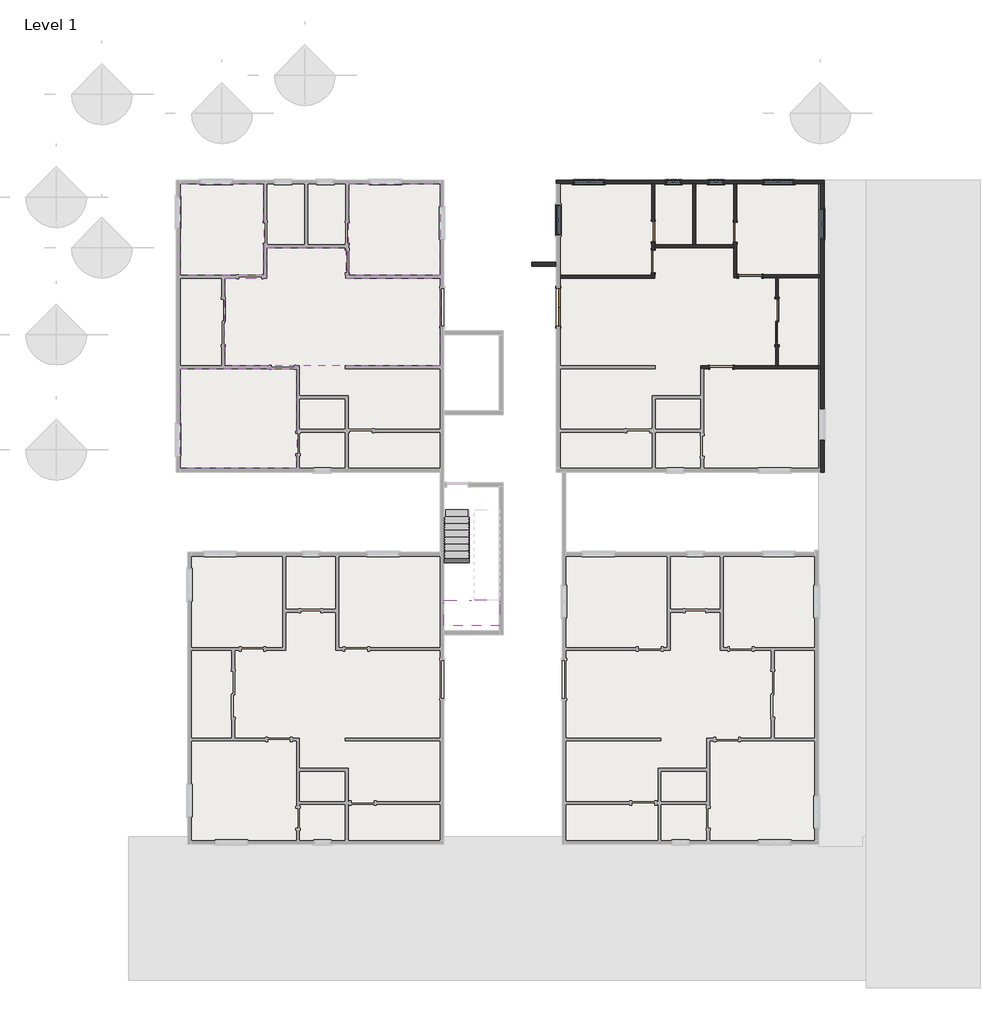
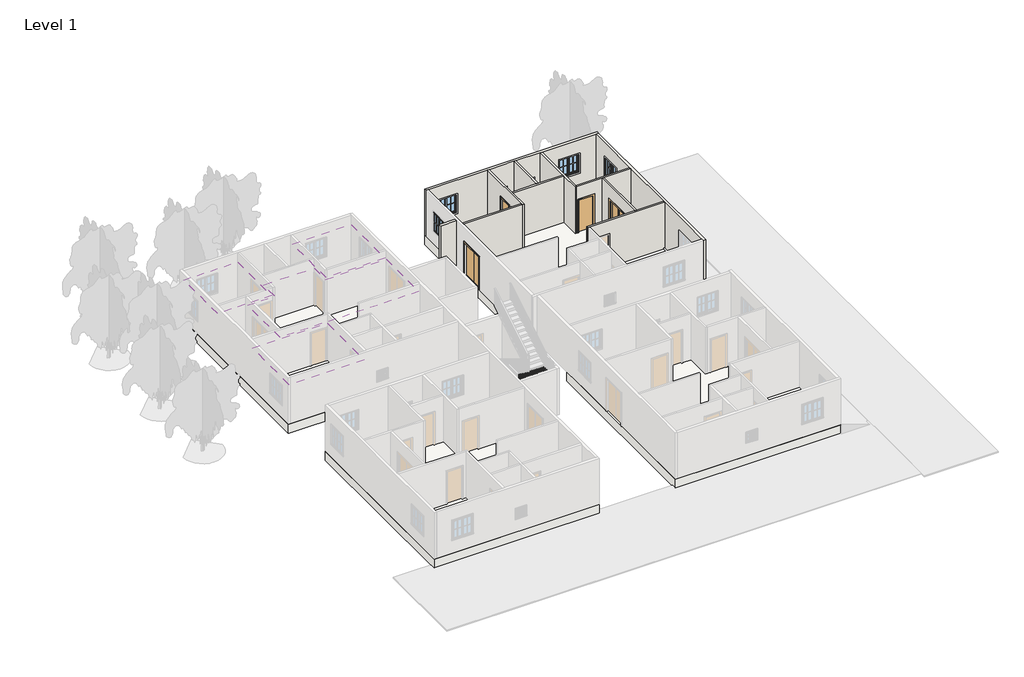
# One storey, part 3 of 7: 11 walls, 6 doors, 6 windows, 4 coverings, 2 slabs, 1 stair flight.
"""IFC4 building model written with IfcOpenShell, lengths in millimetres."""

from ifc_helpers import new_model, si_unit, point, frame, frame_2d, origin, origin_with_axes, place, context, project, spatial, polyline, circle_curve, trimmed, segment, composite_curve, outline, extrude, faceted_brep, transform, mapped, element, save
from components import door_a09c2f77, door_166d4031, door_d141acb4, door_e5f9f3c4, window_0c121b81, window_191d0cfb

model = new_model("IFC4")

# Units and contexts
model_context = context("Model", 3, world=origin())
ifc_project = project(units=[si_unit("LENGTHUNIT", "METRE", prefix="MILLI")], contexts=[model_context])

# Site, building, storey
site = spatial("IfcSite", under=ifc_project)
building = spatial("IfcBuilding", under=site)
storey = spatial("IfcBuildingStorey", under=building, Name="Level 1", Elevation=0.0)

# Coverings
placement = place(None, origin())
element("IfcCovering", 1, ObjectType="2' x 4' ACT System", at=placement, inside=storey, context=model_context, shape_type="SweptSolid", body=[
    extrude(outline(polyline([(-14056.8844485, 6278.5935985), (-9395.9844485, 6278.5935985), (-9395.9844485, 2290.7935985), (-14056.8844485, 2290.7935985), (-14056.8844485, 6278.5935985)]), holes=[polyline([(-13599.6844485, 5668.9935985), (-13599.6844485, 2747.9935985), (-10005.5844485, 2747.9935985), (-10005.5844485, 5668.9935985), (-13599.6844485, 5668.9935985)])]), frame((0.0, 0.0, 2438.4), z_axis=(0.0, 0.0, 1.0), x_axis=(1.0, 0.0, 0.0)), (0.0, 0.0, 1.0), 57.15),
    extrude(outline(composite_curve([segment(trimmed(circle_curve(frame_2d((-11892.8240227, 4343.2390508)), 863.6), [point((-12756.4240227, 4343.2390508))], [point((-11029.2240227, 4343.2390508))], False, "CARTESIAN"), True, "CONTINUOUS"), segment(trimmed(circle_curve(frame_2d((-11892.8240227, 4343.2390508)), 863.6), [point((-11029.2240227, 4343.2390508))], [point((-12756.4240227, 4343.2390508))], False, "CARTESIAN"), True, "CONTINUOUS")], self_intersect=False), holes=[composite_curve([segment(trimmed(circle_curve(frame_2d((-11892.8240227, 4343.2390508)), 660.4), [point((-12553.2240227, 4343.2390508))], [point((-11232.4240227, 4343.2390508))], True, "CARTESIAN"), True, "CONTINUOUS"), segment(trimmed(circle_curve(frame_2d((-11892.8240227, 4343.2390508)), 660.4), [point((-11232.4240227, 4343.2390508))], [point((-12553.2240227, 4343.2390508))], True, "CARTESIAN"), True, "CONTINUOUS")], self_intersect=False)]), frame((0.0, 0.0, 2438.4), z_axis=(0.0, 0.0, 1.0), x_axis=(1.0, 0.0, 0.0)), (0.0, 0.0, 1.0), 57.15),
])
element("IfcCovering", 2, ObjectType="2' x 4' ACT System", at=placement, inside=storey, context=model_context, shape_type="SweptSolid", body=[
    extrude(outline(polyline([(-14056.8844485, 13669.9935985), (-10704.0844485, 13669.9935985), (-10704.0844485, 10012.3935985), (-14056.8844485, 10012.3935985), (-14056.8844485, 13669.9935985)]), holes=[polyline([(-13447.2844485, 13060.3935985), (-13447.2844485, 10621.9935985), (-11313.6844485, 10621.9935985), (-11313.6844485, 13060.3935985), (-13447.2844485, 13060.3935985)])]), frame((0.0, 0.0, 2438.4), z_axis=(0.0, 0.0, 1.0), x_axis=(1.0, 0.0, 0.0)), (0.0, 0.0, 1.0), 57.15),
])
element("IfcCovering", 3, ObjectType="2' x 4' ACT System", at=placement, inside=storey, context=model_context, shape_type="SweptSolid", body=[
    extrude(outline(polyline([(-7313.1844485, 13669.9935985), (-3655.5844485, 13669.9935985), (-3655.5844485, 10012.3935985), (-7313.1844485, 10012.3935985), (-7313.1844485, 13669.9935985)]), holes=[polyline([(-6703.5844485, 13060.3935985), (-6703.5844485, 10621.9935985), (-4265.1844485, 10621.9935985), (-4265.1844485, 13060.3935985), (-6703.5844485, 13060.3935985)])]), frame((0.0, 0.0, 2438.4), z_axis=(0.0, 0.0, 1.0), x_axis=(1.0, 0.0, 0.0)), (0.0, 0.0, 1.0), 57.15),
    extrude(outline(composite_curve([segment(trimmed(circle_curve(frame_2d((-5588.9279628, 11831.416679)), 762.0), [point((-6350.9279628, 11831.416679))], [point((-4826.9279628, 11831.416679))], False, "CARTESIAN"), True, "CONTINUOUS"), segment(trimmed(circle_curve(frame_2d((-5588.9279628, 11831.416679)), 762.0), [point((-4826.9279628, 11831.416679))], [point((-6350.9279628, 11831.416679))], False, "CARTESIAN"), True, "CONTINUOUS")], self_intersect=False), holes=[composite_curve([segment(trimmed(circle_curve(frame_2d((-5588.9279628, 11831.416679)), 660.4), [point((-6249.3279628, 11831.416679))], [point((-4928.5279628, 11831.416679))], True, "CARTESIAN"), True, "CONTINUOUS"), segment(trimmed(circle_curve(frame_2d((-5588.9279628, 11831.416679)), 660.4), [point((-4928.5279628, 11831.416679))], [point((-6249.3279628, 11831.416679))], True, "CARTESIAN"), True, "CONTINUOUS")], self_intersect=False)]), frame((0.0, 0.0, 2438.4), z_axis=(0.0, 0.0, 1.0), x_axis=(1.0, 0.0, 0.0)), (0.0, 0.0, 1.0), 57.15),
])
element("IfcCovering", 4, ObjectType="2' x 4' ACT System", at=placement, inside=storey, context=model_context, shape_type="SweptSolid", body=[
    extrude(outline(polyline([(-7427.4844485, 11117.2935985), (-7427.4844485, 9898.0935985), (-3655.5844485, 9898.0935985), (-3655.5844485, 6392.8935985), (-12266.1844485, 6392.8935985), (-12266.1844485, 9898.0935985), (-10589.7844485, 9898.0935985), (-10589.7844485, 11117.2935985), (-7427.4844485, 11117.2935985)]), holes=[polyline([(-9980.1844485, 10507.6935985), (-9980.1844485, 9288.4935985), (-11656.5844485, 9288.4935985), (-11656.5844485, 7002.4935985), (-4265.1844485, 7002.4935985), (-4265.1844485, 9288.4935985), (-8037.0844485, 9288.4935985), (-8037.0844485, 10507.6935985), (-9980.1844485, 10507.6935985)])]), frame((0.0, 0.0, 2438.4), z_axis=(0.0, 0.0, 1.0), x_axis=(1.0, 0.0, 0.0)), (0.0, 0.0, 1.0), 57.15),
])

# Doors
door_shape = door_a09c2f77(model_context)
element("IfcDoor", 5, ObjectType="Door-Double-Flush_Panel : 60\" x 84\"", at=placement, inside=storey, context=model_context, shape_type="MappedRepresentation", body=[
    mapped(door_shape, transform((1068.9014317, 8736.0435985, 0.0), x_axis=(0.0, -1.0, 0.0), y_axis=(1.0, 0.0, 0.0), z_axis=(0.0, 0.0, 1.0))),
])
door_2_shape = door_166d4031(model_context)
element("IfcDoor", 6, ObjectType="Door-Double-Sliding : 72\" x 84\"", at=placement, inside=storey, context=model_context, shape_type="MappedRepresentation", body=[
    mapped(door_2_shape, transform((9685.8514317, 8151.8435985, 0.0), x_axis=(0.0, -1.0, 0.0), y_axis=(1.0, 0.0, 0.0), z_axis=(0.0, 0.0, 1.0))),
])
door_3_shape = door_d141acb4(model_context)
element("IfcDoor", 7, ObjectType="Single-Flush : 32\" x 84\"", at=placement, inside=storey, context=model_context, shape_type="MappedRepresentation", body=[
    mapped(door_3_shape, transform((8136.4514317, 11733.2435985, 0.0), x_axis=(0.0, 1.0, 0.0), y_axis=(-1.0, 0.0, 0.0), z_axis=(0.0, 0.0, 1.0))),
])
element("IfcDoor", 8, ObjectType="Single-Flush : 32\" x 84\"", at=placement, inside=storey, context=model_context, shape_type="MappedRepresentation", body=[
    mapped(door_3_shape, transform((4859.8514317, 11758.6435985, 0.0), x_axis=(0.0, -1.0, 0.0), y_axis=(1.0, 0.0, 0.0), z_axis=(0.0, 0.0, 1.0))),
])
door_4_shape = door_e5f9f3c4(model_context)
element("IfcDoor", 9, ObjectType="Single-Flush : 36\" x 84\"", at=placement, inside=storey, context=model_context, shape_type="MappedRepresentation", body=[
    mapped(door_4_shape, transform((4859.8514317, 10564.8435985, 0.0), x_axis=(0.0, 1.0, 0.0), y_axis=(-1.0, 0.0, 0.0), z_axis=(0.0, 0.0, 1.0))),
])
element("IfcDoor", 10, ObjectType="Single-Flush : 36\" x 84\"", at=placement, inside=storey, context=model_context, shape_type="MappedRepresentation", body=[
    mapped(door_4_shape, transform((8746.0514317, 9967.9435985, 0.0), x_axis=(1.0, 0.0, 0.0), y_axis=(0.0, 1.0, 0.0), z_axis=(0.0, 0.0, 1.0))),
])

# Slabs
element("IfcSlab", 11, ObjectType="7\" Thickness", at=placement, inside=storey, context=model_context, shape_type="Brep", body=[
    faceted_brep([(-3503.1844485, -4001.8730729, 2370.6666667), (-1267.9844485, -4001.8730729, 2370.6666667), (-1267.9844485, -3137.6775611, 2370.6666667), (-1267.9844485, -2985.8730729, 2370.6666667), (-1267.9844485, -2966.8230729, 2370.6666667), (-2283.9844485, -2966.8230729, 2370.6666667), (-2283.9844485, -2985.8730729, 2370.6666667), (-2487.1844485, -2985.8730729, 2370.6666667), (-3503.1844485, -2985.8730729, 2370.6666667), (-3503.1844485, -3113.4685846, 2370.6666667), (-2487.1844485, -3004.9230729, 2201.3333333), (-2487.1844485, -2985.8730729, 2192.8666667), (-2487.1844485, -3004.9230729, 2192.8666667), (-3503.1844485, -3004.9230729, 2201.3333333), (-2487.1844485, -3004.9230729, 2127.081508), (-3503.1844485, -3004.9230729, 2127.081508), (-3503.1844485, -3113.4685846, 2192.8666667), (-3503.1844485, -4001.8730729, 2192.8666667), (-1267.9844485, -4001.8730729, 2192.8666667), (-1267.9844485, -3137.6775611, 2192.8666667), (-1267.9844485, -2985.8730729, 2284.8693868), (-1267.9844485, -2966.8230729, 2296.4148413), (-2283.9844485, -2966.8230729, 2296.4148413), (-2283.9844485, -2985.8730729, 2284.8693868), (-2283.9844485, -2985.8730729, 2192.8666667), (-2283.9844485, -3137.6775611, 2192.8666667), (-2487.1844485, -3113.4685846, 2192.8666667)], [[[0, 1, 2, 3, 4, 5, 6, 7, 8, 9]], [[10, 7, 11, 12]], [[13, 10, 12, 14, 15]], [[8, 13, 15, 16, 17, 0, 9]], [[1, 0, 17, 18]], [[1, 18, 19, 20, 3, 2]], [[4, 3, 20, 21]], [[5, 4, 21, 22]], [[6, 5, 22, 23]], [[7, 6, 23, 24, 11]], [[8, 7, 10, 13]], [[24, 25, 19, 18, 17, 16, 26, 12, 11]], [[25, 24, 23]], [[26, 16, 15, 14]], [[12, 26, 14]], [[19, 25, 23, 22, 21, 20]]]),
])
element("IfcSlab", 12, ObjectType="FLOOR", at=placement, inside=storey, context=model_context, shape_type="SweptSolid", body=[
    extrude(outline(polyline([(-14209.2844485, 13822.3935985), (-3503.1844485, 13822.3935985), (-3503.1844485, 2138.3935985), (-14209.2844485, 2138.3935985), (-14209.2844485, 13822.3935985)])), frame((0.0, 0.0, -609.6), z_axis=(0.0, 0.0, 1.0), x_axis=(1.0, 0.0, 0.0)), (0.0, 0.0, 1.0), 609.6),
    extrude(outline(polyline([(-13756.5663899, -1055.4730729), (-3503.1844485, -1055.4730729), (-3503.1844485, -12746.0064015), (-13756.5663899, -12746.0064015), (-13756.5663899, -1055.4730729)])), frame((0.0, 0.0, -609.6), z_axis=(0.0, 0.0, 1.0), x_axis=(1.0, 0.0, 0.0)), (0.0, 0.0, 1.0), 609.6),
    extrude(outline(polyline([(1221.2155515, -1055.4730729), (11475.1785285, -1055.4730729), (11475.1785285, -12746.0064015), (1221.2155515, -12746.0064015), (1221.2155515, -1055.4730729)])), frame((0.0, 0.0, -609.6), z_axis=(0.0, 0.0, 1.0), x_axis=(1.0, 0.0, 0.0)), (0.0, 0.0, 1.0), 609.6),
    extrude(outline(polyline([(992.7014317, 13822.3935985), (11698.8014317, 13822.3935985), (11698.8014317, 2138.3935985), (992.7014317, 2138.3935985), (992.7014317, 13822.3935985)])), frame((0.0, 0.0, -609.6), z_axis=(0.0, 0.0, 1.0), x_axis=(1.0, 0.0, 0.0)), (0.0, 0.0, 1.0), 609.6),
])

# Stair flight
element("IfcStairFlight", 13, ObjectType="3/4\" Nosing", at=placement, inside=storey, context=model_context, shape_type="Brep", body=[
    faceted_brep([(-2487.1844485, 646.3269271, 169.3333333), (-3503.1844485, 646.3269271, 169.3333333), (-3503.1844485, 347.8769271, 169.3333333), (-2487.1844485, 347.8769271, 169.3333333), (-2487.1844485, 347.8769271, 95.081508), (-2487.1844485, 504.7614154, 0.0), (-2487.1844485, 627.2769271, 0.0), (-3503.1844485, 627.2769271, 0.0), (-3503.1844485, 504.7614154, 0.0), (-3503.1844485, 347.8769271, 95.081508), (-2487.1844485, 366.9269271, 338.6666667), (-3503.1844485, 366.9269271, 338.6666667), (-3503.1844485, 68.4769271, 338.6666667), (-2487.1844485, 68.4769271, 338.6666667), (-2487.1844485, 68.4769271, 264.4148413), (-3503.1844485, 68.4769271, 264.4148413), (-2487.1844485, 87.5269271, 508.0), (-3503.1844485, 87.5269271, 508.0), (-3503.1844485, -210.9230729, 508.0), (-2487.1844485, -210.9230729, 508.0), (-2487.1844485, -210.9230729, 433.7481747), (-3503.1844485, -210.9230729, 433.7481747), (-2487.1844485, -191.8730729, 677.3333333), (-3503.1844485, -191.8730729, 677.3333333), (-3503.1844485, -490.3230729, 677.3333333), (-2487.1844485, -490.3230729, 677.3333333), (-2487.1844485, -490.3230729, 603.081508), (-3503.1844485, -490.3230729, 603.081508), (-2487.1844485, -471.2730729, 846.6666667), (-3503.1844485, -471.2730729, 846.6666667), (-3503.1844485, -769.7230729, 846.6666667), (-2487.1844485, -769.7230729, 846.6666667), (-2487.1844485, -769.7230729, 772.4148413), (-3503.1844485, -769.7230729, 772.4148413), (-2487.1844485, -750.6730729, 1016.0), (-3503.1844485, -750.6730729, 1016.0), (-3503.1844485, -1049.1230729, 1016.0), (-2487.1844485, -1049.1230729, 1016.0), (-2487.1844485, -1049.1230729, 941.7481747), (-3503.1844485, -1049.1230729, 941.7481747), (-2487.1844485, -1030.0730729, 1185.3333333), (-3503.1844485, -1030.0730729, 1185.3333333), (-3503.1844485, -1328.5230729, 1185.3333333), (-2487.1844485, -1328.5230729, 1185.3333333), (-2487.1844485, -1328.5230729, 1111.081508), (-3503.1844485, -1328.5230729, 1111.081508), (-2487.1844485, -1309.4730729, 1354.6666667), (-3503.1844485, -1309.4730729, 1354.6666667), (-3503.1844485, -1607.9230729, 1354.6666667), (-2487.1844485, -1607.9230729, 1354.6666667), (-2487.1844485, -1607.9230729, 1280.4148413), (-3503.1844485, -1607.9230729, 1280.4148413), (-2487.1844485, -1588.8730729, 1524.0), (-3503.1844485, -1588.8730729, 1524.0), (-3503.1844485, -1887.3230729, 1524.0), (-2487.1844485, -1887.3230729, 1524.0), (-2487.1844485, -1887.3230729, 1449.7481747), (-3503.1844485, -1887.3230729, 1449.7481747), (-2487.1844485, -1868.2730729, 1693.3333333), (-3503.1844485, -1868.2730729, 1693.3333333), (-3503.1844485, -2166.7230729, 1693.3333333), (-2487.1844485, -2166.7230729, 1693.3333333), (-2487.1844485, -2166.7230729, 1619.081508), (-3503.1844485, -2166.7230729, 1619.081508), (-2487.1844485, -2147.6730729, 1862.6666667), (-3503.1844485, -2147.6730729, 1862.6666667), (-3503.1844485, -2446.1230729, 1862.6666667), (-2487.1844485, -2446.1230729, 1862.6666667), (-2487.1844485, -2446.1230729, 1788.4148413), (-3503.1844485, -2446.1230729, 1788.4148413), (-2487.1844485, -2427.0730729, 2032.0), (-3503.1844485, -2427.0730729, 2032.0), (-3503.1844485, -2725.5230729, 2032.0), (-2487.1844485, -2725.5230729, 2032.0), (-2487.1844485, -2725.5230729, 1957.7481747), (-3503.1844485, -2725.5230729, 1957.7481747), (-2487.1844485, -2706.4730729, 2201.3333333), (-3503.1844485, -2706.4730729, 2201.3333333), (-3503.1844485, -2985.8730729, 2201.3333333), (-3503.1844485, -3004.9230729, 2201.3333333), (-2487.1844485, -3004.9230729, 2201.3333333), (-2487.1844485, -2985.8730729, 2201.3333333), (-2487.1844485, -3004.9230729, 2192.8666667), (-2487.1844485, -3004.9230729, 2127.081508), (-3503.1844485, -2985.8730729, 2115.5360535), (-3503.1844485, -3004.9230729, 2127.081508)], [[[0, 1, 2, 3]], [[0, 3, 4, 5, 6]], [[2, 1, 7, 8, 9]], [[10, 11, 12, 13]], [[10, 13, 14, 4, 3]], [[12, 11, 2, 9, 15]], [[16, 17, 18, 19]], [[16, 19, 20, 14, 13]], [[18, 17, 12, 15, 21]], [[22, 23, 24, 25]], [[22, 25, 26, 20, 19]], [[24, 23, 18, 21, 27]], [[28, 29, 30, 31]], [[28, 31, 32, 26, 25]], [[30, 29, 24, 27, 33]], [[34, 35, 36, 37]], [[34, 37, 38, 32, 31]], [[36, 35, 30, 33, 39]], [[40, 41, 42, 43]], [[40, 43, 44, 38, 37]], [[42, 41, 36, 39, 45]], [[46, 47, 48, 49]], [[46, 49, 50, 44, 43]], [[48, 47, 42, 45, 51]], [[52, 53, 54, 55]], [[52, 55, 56, 50, 49]], [[54, 53, 48, 51, 57]], [[58, 59, 60, 61]], [[58, 61, 62, 56, 55]], [[60, 59, 54, 57, 63]], [[64, 65, 66, 67]], [[64, 67, 68, 62, 61]], [[66, 65, 60, 63, 69]], [[70, 71, 72, 73]], [[70, 73, 74, 68, 67]], [[72, 71, 66, 69, 75]], [[76, 77, 78, 79, 80, 81]], [[73, 76, 81, 80, 82, 83, 74]], [[78, 77, 72, 75, 84]], [[79, 78, 84, 85]], [[80, 79, 85, 83, 82]], [[1, 0, 6, 7]], [[3, 2, 11, 10]], [[13, 12, 17, 16]], [[19, 18, 23, 22]], [[25, 24, 29, 28]], [[31, 30, 35, 34]], [[37, 36, 41, 40]], [[43, 42, 47, 46]], [[49, 48, 53, 52]], [[55, 54, 59, 58]], [[61, 60, 65, 64]], [[67, 66, 71, 70]], [[73, 72, 77, 76]], [[7, 6, 5, 8]], [[8, 5, 4, 14, 20, 26, 32, 38, 44, 50, 56, 62, 68, 74, 83, 85, 84, 75, 69, 63, 57, 51, 45, 39, 33, 27, 21, 15, 9]]]),
])

# Walls
element("IfcWall", 14, ObjectType="4.5\"", at=placement, inside=storey, context=model_context, shape_type="Brep", body=[
    faceted_brep([(4802.7014317, 11352.2435985, 2133.6), (4802.7014317, 11352.2435985, 0.0), (4802.7014317, 11022.0435985, 0.0), (4802.7014317, 11022.0435985, 2133.6), (4802.7014317, 10107.6435985, 2133.6), (4802.7014317, 10107.6435985, 0.0), (4802.7014317, 10012.3935985, 0.0), (4802.7014317, 9898.0935985, 0.0), (4802.7014317, 9898.0935985, 3048.0), (4802.7014317, 10012.3935985, 3048.0), (4802.7014317, 13669.9935985, 3048.0), (4802.7014317, 13669.9935985, 0.0), (4802.7014317, 12165.0435985, 0.0), (4802.7014317, 12165.0435985, 2133.6), (4917.0014317, 11022.0435985, 0.0), (4917.0014317, 11117.2935985, 0.0), (4917.0014317, 11231.5935985, 0.0), (4917.0014317, 11352.2435985, 0.0), (4917.0014317, 11352.2435985, 2133.6), (4917.0014317, 12165.0435985, 2133.6), (4917.0014317, 12165.0435985, 0.0), (4917.0014317, 13669.9935985, 0.0), (4917.0014317, 13669.9935985, 3048.0), (4917.0014317, 11231.5935985, 3048.0), (4917.0014317, 11117.2935985, 3048.0), (4917.0014317, 9898.0935985, 3048.0), (4917.0014317, 9898.0935985, 0.0), (4917.0014317, 10107.6435985, 0.0), (4917.0014317, 10107.6435985, 2133.6), (4917.0014317, 11022.0435985, 2133.6)], [[[0, 1, 2, 3, 4, 5, 6, 7, 8, 9, 10, 11, 12, 13]], [[14, 15, 16, 17, 18, 19, 20, 21, 22, 23, 24, 25, 26, 27, 28, 29]], [[27, 26, 7, 6, 5]], [[12, 11, 21, 20]], [[2, 1, 17, 16, 15, 14]], [[11, 10, 22, 21]], [[8, 7, 26, 25]], [[3, 2, 14, 29]], [[4, 3, 29, 28]], [[5, 4, 28, 27]], [[18, 17, 1, 0]], [[19, 18, 0, 13]], [[20, 19, 13, 12]], [[10, 9, 8, 25, 24, 23, 22]]]),
])
element("IfcWall", 15, ObjectType="4.5\"", at=placement, inside=storey, context=model_context, shape_type="SweptSolid", body=[
    extrude(outline(polyline([(1145.1014317, 10012.3935985), (4802.7014317, 10012.3935985), (4802.7014317, 9898.0935985), (1145.1014317, 9898.0935985), (1145.1014317, 10012.3935985)])), origin_with_axes(), (0.0, 0.0, 1.0), 3048.0),
])
element("IfcWall", 16, ObjectType="4.5\"", at=placement, inside=storey, context=model_context, shape_type="Brep", body=[
    faceted_brep([(4917.0014317, 11117.2935985, 0.0), (8079.3014317, 11117.2935985, 0.0), (8079.3014317, 11117.2935985, 3048.0), (4917.0014317, 11117.2935985, 3048.0), (4917.0014317, 11231.5935985, 0.0), (4917.0014317, 11231.5935985, 3048.0), (6441.0014317, 11231.5935985, 3048.0), (6555.3014317, 11231.5935985, 3048.0), (8079.3014317, 11231.5935985, 3048.0), (8079.3014317, 11231.5935985, 0.0), (6555.3014317, 11231.5935985, 0.0), (6441.0014317, 11231.5935985, 0.0)], [[[0, 1, 2, 3]], [[4, 5, 6, 7, 8, 9, 10, 11]], [[1, 0, 4, 11, 10, 9]], [[0, 3, 5, 4]], [[2, 1, 9, 8]], [[3, 2, 8, 7, 6, 5]]]),
])
element("IfcWall", 17, ObjectType="4.5\"", at=placement, inside=storey, context=model_context, shape_type="SweptSolid", body=[
    extrude(outline(polyline([(6441.0014317, 11231.5935985), (6441.0014317, 13669.9935985), (6555.3014317, 13669.9935985), (6555.3014317, 11231.5935985), (6441.0014317, 11231.5935985)])), origin_with_axes(), (0.0, 0.0, 1.0), 3048.0),
])
element("IfcWall", 18, ObjectType="4.5\"", at=placement, inside=storey, context=model_context, shape_type="Brep", body=[
    faceted_brep([(8079.3014317, 13669.9935985, 0.0), (8079.3014317, 12139.6435985, 0.0), (8079.3014317, 12139.6435985, 2133.6), (8079.3014317, 11326.8435985, 2133.6), (8079.3014317, 11326.8435985, 0.0), (8079.3014317, 11231.5935985, 0.0), (8079.3014317, 11117.2935985, 0.0), (8079.3014317, 9910.7935985, 0.0), (8079.3014317, 9910.7935985, 3048.0), (8079.3014317, 11117.2935985, 3048.0), (8079.3014317, 11231.5935985, 3048.0), (8079.3014317, 13669.9935985, 3048.0), (8193.6014317, 12139.6435985, 2133.6), (8193.6014317, 12139.6435985, 0.0), (8193.6014317, 13669.9935985, 0.0), (8193.6014317, 13669.9935985, 3048.0), (8193.6014317, 10025.0935985, 3048.0), (8193.6014317, 9910.7935985, 3048.0), (8193.6014317, 9910.7935985, 0.0), (8193.6014317, 10025.0935985, 0.0), (8193.6014317, 11326.8435985, 0.0), (8193.6014317, 11326.8435985, 2133.6)], [[[0, 1, 2, 3, 4, 5, 6, 7, 8, 9, 10, 11]], [[12, 13, 14, 15, 16, 17, 18, 19, 20, 21]], [[14, 13, 1, 0]], [[20, 19, 18, 7, 6, 5, 4]], [[0, 11, 15, 14]], [[8, 7, 18, 17]], [[2, 1, 13, 12]], [[3, 2, 12, 21]], [[4, 3, 21, 20]], [[11, 10, 9, 8, 17, 16, 15]]]),
])
element("IfcWall", 19, ObjectType="4.5\"", at=placement, inside=storey, context=model_context, shape_type="Brep", body=[
    faceted_brep([(9203.2514317, 9910.7935985, 2133.6), (9203.2514317, 9910.7935985, 0.0), (9755.7014317, 9910.7935985, 0.0), (9870.0014317, 9910.7935985, 0.0), (11546.4014317, 9910.7935985, 0.0), (11546.4014317, 9910.7935985, 3048.0), (9870.0014317, 9910.7935985, 3048.0), (9755.7014317, 9910.7935985, 3048.0), (8193.6014317, 9910.7935985, 3048.0), (8193.6014317, 9910.7935985, 0.0), (8288.8514317, 9910.7935985, 0.0), (8288.8514317, 9910.7935985, 2133.6), (11546.4014317, 10025.0935985, 0.0), (9203.2514317, 10025.0935985, 0.0), (9203.2514317, 10025.0935985, 2133.6), (8288.8514317, 10025.0935985, 2133.6), (8288.8514317, 10025.0935985, 0.0), (8193.6014317, 10025.0935985, 0.0), (8193.6014317, 10025.0935985, 3048.0), (11546.4014317, 10025.0935985, 3048.0)], [[[0, 1, 2, 3, 4, 5, 6, 7, 8, 9, 10, 11]], [[12, 13, 14, 15, 16, 17, 18, 19]], [[10, 9, 17, 16]], [[4, 3, 2, 1, 13, 12]], [[9, 8, 18, 17]], [[5, 4, 12, 19]], [[14, 13, 1, 0]], [[15, 14, 0, 11]], [[16, 15, 11, 10]], [[8, 7, 6, 5, 19, 18]]]),
])
element("IfcWall", 20, ObjectType="4.5\"", at=placement, inside=storey, context=model_context, shape_type="SweptSolid", body=[
    extrude(outline(polyline([(7237.4435985, 2133.6), (7237.4435985, 0.0), (6392.8935985, 0.0), (6392.8935985, 3048.0), (9910.7935985, 3048.0), (9910.7935985, 0.0), (9066.2435985, 0.0), (9066.2435985, 2133.6), (7237.4435985, 2133.6)])), frame((9755.7014317, 0.0, 0.0), z_axis=(1.0, 0.0, 0.0), x_axis=(0.0, 1.0, 0.0)), (0.0, 0.0, 1.0), 114.3),
])
element("IfcWall", 21, ObjectType="4.5\"", at=placement, inside=storey, context=model_context, shape_type="Brep", body=[
    faceted_brep([(11546.4014317, 6392.8935985, 0.0), (9870.0014317, 6392.8935985, 0.0), (9755.7014317, 6392.8935985, 0.0), (8047.5514317, 6392.8935985, 0.0), (8047.5514317, 6392.8935985, 2133.6), (7133.1514317, 6392.8935985, 2133.6), (7133.1514317, 6392.8935985, 0.0), (6771.2014317, 6392.8935985, 0.0), (6771.2014317, 6392.8935985, 3048.0), (9755.7014317, 6392.8935985, 3048.0), (9870.0014317, 6392.8935985, 3048.0), (11546.4014317, 6392.8935985, 3048.0), (8047.5514317, 6278.5935985, 2133.6), (8047.5514317, 6278.5935985, 0.0), (11546.4014317, 6278.5935985, 0.0), (11546.4014317, 6278.5935985, 3048.0), (6885.5014317, 6278.5935985, 3048.0), (6771.2014317, 6278.5935985, 3048.0), (6771.2014317, 6278.5935985, 0.0), (6885.5014317, 6278.5935985, 0.0), (7133.1514317, 6278.5935985, 0.0), (7133.1514317, 6278.5935985, 2133.6)], [[[0, 1, 2, 3, 4, 5, 6, 7, 8, 9, 10, 11]], [[12, 13, 14, 15, 16, 17, 18, 19, 20, 21]], [[14, 13, 3, 2, 1, 0]], [[20, 19, 18, 7, 6]], [[0, 11, 15, 14]], [[8, 7, 18, 17]], [[4, 3, 13, 12]], [[5, 4, 12, 21]], [[6, 5, 21, 20]], [[11, 10, 9, 8, 17, 16, 15]]]),
])
element("IfcWall", 22, ObjectType="6\"", at=placement, inside=storey, context=model_context, shape_type="Brep", body=[
    faceted_brep([(992.7014317, 13669.9935985, 0.0), (1145.1014317, 13669.9935985, 0.0), (4802.7014317, 13669.9935985, 0.0), (4917.0014317, 13669.9935985, 0.0), (6441.0014317, 13669.9935985, 0.0), (6555.3014317, 13669.9935985, 0.0), (8079.3014317, 13669.9935985, 0.0), (8193.6014317, 13669.9935985, 0.0), (11546.4014317, 13669.9935985, 0.0), (11698.8014317, 13669.9935985, 0.0), (11698.8014317, 13669.9935985, 3048.0), (11546.4014317, 13669.9935985, 3048.0), (8193.6014317, 13669.9935985, 3048.0), (8079.3014317, 13669.9935985, 3048.0), (6555.3014317, 13669.9935985, 3048.0), (6441.0014317, 13669.9935985, 3048.0), (4917.0014317, 13669.9935985, 3048.0), (4802.7014317, 13669.9935985, 3048.0), (1145.1014317, 13669.9935985, 3048.0), (992.7014317, 13669.9935985, 3048.0), (2897.7014317, 13669.9935985, 2133.6), (2897.7014317, 13669.9935985, 914.4), (1678.5014317, 13669.9935985, 914.4), (1678.5014317, 13669.9935985, 2133.6), (10489.1264317, 13669.9935985, 2133.6), (10489.1264317, 13669.9935985, 914.4), (9269.9264317, 13669.9935985, 914.4), (9269.9264317, 13669.9935985, 2133.6), (5983.8014317, 13669.9935985, 1524.0), (5983.8014317, 13669.9935985, 914.4), (5374.2014317, 13669.9935985, 914.4), (5374.2014317, 13669.9935985, 1524.0), (7679.2514317, 13669.9935985, 1524.0), (7679.2514317, 13669.9935985, 914.4), (7069.6514317, 13669.9935985, 914.4), (7069.6514317, 13669.9935985, 1524.0), (992.7014317, 13822.3935985, 0.0), (992.7014317, 13822.3935985, 3048.0), (11698.8014317, 13822.3935985, 3048.0), (11698.8014317, 13822.3935985, 0.0), (2897.7014317, 13822.3935985, 2133.6), (1678.5014317, 13822.3935985, 2133.6), (1678.5014317, 13822.3935985, 914.4), (2897.7014317, 13822.3935985, 914.4), (10489.1264317, 13822.3935985, 2133.6), (9269.9264317, 13822.3935985, 2133.6), (9269.9264317, 13822.3935985, 914.4), (10489.1264317, 13822.3935985, 914.4), (5983.8014317, 13822.3935985, 1524.0), (5374.2014317, 13822.3935985, 1524.0), (5374.2014317, 13822.3935985, 914.4), (5983.8014317, 13822.3935985, 914.4), (7679.2514317, 13822.3935985, 1524.0), (7069.6514317, 13822.3935985, 1524.0), (7069.6514317, 13822.3935985, 914.4), (7679.2514317, 13822.3935985, 914.4)], [[[0, 1, 2, 3, 4, 5, 6, 7, 8, 9, 10, 11, 12, 13, 14, 15, 16, 17, 18, 19], [20, 21, 22, 23], [24, 25, 26, 27], [28, 29, 30, 31], [32, 33, 34, 35]], [[36, 37, 38, 39], [40, 41, 42, 43], [44, 45, 46, 47], [48, 49, 50, 51], [52, 53, 54, 55]], [[9, 8, 7, 6, 5, 4, 3, 2, 1, 0, 36, 39]], [[0, 19, 37, 36]], [[10, 9, 39, 38]], [[21, 20, 40, 43]], [[22, 21, 43, 42]], [[23, 22, 42, 41]], [[20, 23, 41, 40]], [[25, 24, 44, 47]], [[26, 25, 47, 46]], [[27, 26, 46, 45]], [[24, 27, 45, 44]], [[29, 28, 48, 51]], [[30, 29, 51, 50]], [[31, 30, 50, 49]], [[28, 31, 49, 48]], [[33, 32, 52, 55]], [[34, 33, 55, 54]], [[35, 34, 54, 53]], [[32, 35, 53, 52]], [[19, 18, 17, 16, 15, 14, 13, 12, 11, 10, 38, 37]]]),
])
element("IfcWall", 23, ObjectType="6\"", at=placement, inside=storey, context=model_context, shape_type="Brep", body=[
    faceted_brep([(11546.4014317, 13669.9935985, 0.0), (11546.4014317, 10025.0935985, 0.0), (11546.4014317, 9910.7935985, 0.0), (11546.4014317, 6392.8935985, 0.0), (11546.4014317, 6278.5935985, 0.0), (11546.4014317, 2290.7935985, 0.0), (11546.4014317, 2138.3935985, 0.0), (11546.4014317, 2138.3935985, 3048.0), (11546.4014317, 2290.7935985, 3048.0), (11546.4014317, 6278.5935985, 3048.0), (11546.4014317, 6392.8935985, 3048.0), (11546.4014317, 9910.7935985, 3048.0), (11546.4014317, 10025.0935985, 3048.0), (11546.4014317, 13669.9935985, 3048.0), (11546.4014317, 11460.1935985, 2133.6), (11546.4014317, 11460.1935985, 914.4), (11546.4014317, 12679.3935985, 914.4), (11546.4014317, 12679.3935985, 2133.6), (11546.4014317, 3433.7935985, 2133.6), (11546.4014317, 3433.7935985, 914.4), (11546.4014317, 4652.9935985, 914.4), (11546.4014317, 4652.9935985, 2133.6), (11698.8014317, 13669.9935985, 0.0), (11698.8014317, 13669.9935985, 3048.0), (11698.8014317, 2138.3935985, 3048.0), (11698.8014317, 2138.3935985, 0.0), (11698.8014317, 11460.1935985, 2133.6), (11698.8014317, 12679.3935985, 2133.6), (11698.8014317, 12679.3935985, 914.4), (11698.8014317, 11460.1935985, 914.4), (11698.8014317, 3433.7935985, 2133.6), (11698.8014317, 4652.9935985, 2133.6), (11698.8014317, 4652.9935985, 914.4), (11698.8014317, 3433.7935985, 914.4)], [[[0, 1, 2, 3, 4, 5, 6, 7, 8, 9, 10, 11, 12, 13], [14, 15, 16, 17], [18, 19, 20, 21]], [[22, 23, 24, 25], [26, 27, 28, 29], [30, 31, 32, 33]], [[6, 5, 4, 3, 2, 1, 0, 22, 25]], [[0, 13, 23, 22]], [[7, 6, 25, 24]], [[15, 14, 26, 29]], [[16, 15, 29, 28]], [[17, 16, 28, 27]], [[14, 17, 27, 26]], [[19, 18, 30, 33]], [[20, 19, 33, 32]], [[21, 20, 32, 31]], [[18, 21, 31, 30]], [[13, 12, 11, 10, 9, 8, 7, 24, 23]]]),
])
element("IfcWall", 24, ObjectType="6\"", at=placement, inside=storey, context=model_context, shape_type="SweptSolid", body=[
    extrude(outline(polyline([(992.7014317, 10383.7917043), (2.1014317, 10383.7917043), (2.1014317, 10536.1917043), (992.7014317, 10536.1917043), (992.7014317, 10383.7917043)])), origin_with_axes(), (0.0, 0.0, 1.0), 3048.0),
])

# Windows
window_shape = window_0c121b81(model_context)
element("IfcWindow", 25, ObjectType="Window-Casement-Double : 24\" x 24\"", at=placement, inside=storey, context=model_context, shape_type="MappedRepresentation", body=[
    mapped(window_shape, transform((5679.0014317, 13746.1935985, 0.0), x_axis=(1.0, 0.0, 0.0), y_axis=(0.0, 1.0, 0.0), z_axis=(0.0, 0.0, 1.0))),
])
element("IfcWindow", 26, ObjectType="Window-Casement-Double : 24\" x 24\"", at=placement, inside=storey, context=model_context, shape_type="MappedRepresentation", body=[
    mapped(window_shape, transform((7374.4514317, 13746.1935985, 0.0), x_axis=(1.0, 0.0, 0.0), y_axis=(0.0, 1.0, 0.0), z_axis=(0.0, 0.0, 1.0))),
])
window_2_shape = window_191d0cfb(model_context)
element("IfcWindow", 27, ObjectType="Window-Casement-Double : 48\" x 48\"", at=placement, inside=storey, context=model_context, shape_type="MappedRepresentation", body=[
    mapped(window_2_shape, transform((1068.9014317, 12222.1935985, 0.0), x_axis=(0.0, 1.0, 0.0), y_axis=(-1.0, 0.0, 0.0), z_axis=(0.0, 0.0, 1.0))),
])
element("IfcWindow", 28, ObjectType="Window-Casement-Double : 48\" x 48\"", at=placement, inside=storey, context=model_context, shape_type="MappedRepresentation", body=[
    mapped(window_2_shape, transform((2288.1014317, 13746.1935985, 0.0), x_axis=(1.0, 0.0, 0.0), y_axis=(0.0, 1.0, 0.0), z_axis=(0.0, 0.0, 1.0))),
])
element("IfcWindow", 29, ObjectType="Window-Casement-Double : 48\" x 48\"", at=placement, inside=storey, context=model_context, shape_type="MappedRepresentation", body=[
    mapped(window_2_shape, transform((9879.5264317, 13746.1935985, 0.0), x_axis=(1.0, 0.0, 0.0), y_axis=(0.0, 1.0, 0.0), z_axis=(0.0, 0.0, 1.0))),
])
element("IfcWindow", 30, ObjectType="Window-Casement-Double : 48\" x 48\"", at=placement, inside=storey, context=model_context, shape_type="MappedRepresentation", body=[
    mapped(window_2_shape, transform((11622.6014317, 12069.7935985, 0.0), x_axis=(0.0, -1.0, 0.0), y_axis=(1.0, 0.0, 0.0), z_axis=(0.0, 0.0, 1.0))),
])

save(model, "model.ifc")

# Revit data of these elements
# Type "2' x 4' ACT System"
#   Assembly Code = "C3030210"
#   built-in parameter 1002203 = 1 (stored number, unit not read)
#   built-in parameter 1002202 = 1 (stored number, unit not read)
#   Layers, outside or top first: 0' - 1 5/8" "Default" (function 1); 0' - 0 5/8" "Acoustic Ceiling Tile 24 x 48" (function 5)
# Type "Door-Double-Flush_Panel : 60\" x 84\""
#   Type Mark = "9"
#   Construction Type Id = "DOOR"
#   Assembly Code = "C1020"
#   Analytic Construction = "Wooden"
#   Thickness = 0' - 2"
#   Thermal Resistance (R) = 2.5876 (h·ft²·°F)/BTU
#   Swing Angle [instance default] = 90.00°
#   Panel Width = 2' - 6"
#   Heat Transfer Coefficient (U) = 0.3865 BTU/(h·ft²·°F)
#   Height = 7' - 0"
#   Trim Projection Ext = 0' - 1"
#   Trim Projection Int = 0' - 1"
#   Trim Width = 0' - 3"
#   Width = 5' - 0"
#   Define Thermal Properties by = 1
#   Panel Material = Wood - Birch - Solid Stained Light Low Gloss
#   Trim Material = Paint - Sienna
#   Visual Light Transmittance = 0
#   Solar Heat Gain Coefficient = 0
#   Function = (empty or 0)
#   Wall Closure = (empty or 0)
# Type "Door-Double-Sliding : 72\" x 84\""
#   Type Mark = "8"
#   Construction Type Id = "opn-d45"
#   Assembly Code = "C1020"
#   Analytic Construction = "Wood frame, double glass door "
#   Thickness = 0' - 2"
#   Thermal Resistance (R) = 1.8150 (h·ft²·°F)/BTU
#   Heat Transfer Coefficient (U) = 0.5510 BTU/(h·ft²·°F)
#   Height = 7' - 0"
#   Rail Width = 0' - 2"
#   Stiles = 0' - 2"
#   Trim Projection Ext = 0' - 1"
#   Trim Projection Int = 0' - 1"
#   Trim Width = 0' - 3"
#   Width = 6' - 0"
#   Define Thermal Properties by = 1
#   Glazing = Glass
#   Panel Material = Wood - Birch - Solid Stained Light Low Gloss
#   Trim Material = Paint - Sienna
#   Visual Light Transmittance = 0
#   Solar Heat Gain Coefficient = 0
#   Function = (empty or 0)
#   Wall Closure = (empty or 0)
# Type "Single-Flush : 32\" x 84\""
#   Type Mark = "3"
#   Construction Type Id = "MDOOR"
#   Assembly Code = "C1020"
#   Analytic Construction = "Metal"
#   Thickness = 0' - 2"
#   Heat Transfer Coefficient (U) = 0.651978 BTU/(h·ft²·°F)
#   Height = 7' - 0"
#   Trim Projection Ext = 0' - 1"
#   Trim Projection Int = 0' - 1"
#   Trim Width = 0' - 3"
#   Width = 2' - 8"
#   Define Thermal Properties by = 1
#   Define Thermal Properties by = 1
#   Door Material = Door - Panel
#   Frame Material = Door - Frame
#   Visual Light Transmittance = 0
#   Solar Heat Gain Coefficient = 0
#   Function = (empty or 0)
#   Wall Closure = (empty or 0)
# Type "Single-Flush : 36\" x 84\""
#   Type Mark = "1"
#   Construction Type Id = "MDOOR"
#   Assembly Code = "C1020"
#   Analytic Construction = "Metal"
#   Thickness = 0' - 2"
#   Heat Transfer Coefficient (U) = 0.651978 BTU/(h·ft²·°F)
#   Height = 7' - 0"
#   Trim Projection Ext = 0' - 1"
#   Trim Projection Int = 0' - 1"
#   Trim Width = 0' - 3"
#   Width = 3' - 0"
#   Define Thermal Properties by = 1
#   Define Thermal Properties by = 1
#   Door Material = Door - Panel
#   Frame Material = Door - Frame
#   Visual Light Transmittance = 0
#   Solar Heat Gain Coefficient = 0
#   Function = (empty or 0)
#   Wall Closure = (empty or 0)
# Type "FLOOR"
#   Assembly Code = "B1010"
#   Function = 0
#   Layers, outside or top first: 2' - 0" "Concrete, Cast-in-Place gray" (function 1)
# Type "4.5\""
#   Assembly Code = "B2010"
#   Layers, outside or top first: 0' - 4 1/2" "4.5\" WALL" (function 1)
# Type "6\""
#   Assembly Code = "B2010"
#   Layers, outside or top first: 0' - 6" "6\" WALL" (function 1)
# Type "Window-Casement-Double : 24\" x 24\""
#   Type Mark = "14"
#   Fire Rating = "0.5h"
#   Assembly Code = "B2020100"
#   Analytic Construction = "Double glazing - domestic"
#   Frame Extension [instance default] = 0' - 0 1/4"
#   Window Inset [instance default] = 0' - 0"
#   Wall Thickness [instance default] = 0' - 6"
#   Interior Wall Closure [instance default] = 0' - 2 1/4"
#   Half Width = 1' - 0"
#   Visual Light Transmittance = 0.81
#   Thermal Resistance (R) = 1.8146 (h·ft²·°F)/BTU
#   Solar Heat Gain Coefficient = 0.76
#   Rough Width = 2' - 0 1/2"
#   Rough Height = 2' - 0 1/2"
#   Height = 2' - 0"
#   Heat Transfer Coefficient (U) = 0.5511 BTU/(h·ft²·°F)
#   Exterior Wall Closure [instance default] = 0' - 1 1/4"
#   Extension Jamb [instance default] = 0' - 2 1/4"
#   Default Sill Height = 3' - 0"
#   Width = 2' - 0"
#   Define Thermal Properties by = 0
#   Muntin Visibility = yes
#   Interior Trim Visibility [instance default] = yes
#   Exterior Trim Visibility [instance default] = yes
#   Extension Jamb Visibility [instance default] = yes
#   Interior Trim Material = Wood - Stained
#   Muntin Pattern = Muntin Pattern_2x2 : Muntin Pattern_2x2
#   Interior Trim = Trim-Window-Interior-Flat : Picture Frame
#   Interior Frame Material = Wood - Stained
#   Glass Panel Material = Glass
#   Exterior Trim Material = Clad - White
#   Exterior Trim = Trim-Window-Exterior-Flat : with Sill
#   Exterior Frame Material = Clad - White
#   Wall Closure = (empty or 0)
# Type "Window-Casement-Double : 48\" x 48\""
#   Type Mark = "16"
#   Fire Rating = "0.5h"
#   Assembly Code = "B2020100"
#   Analytic Construction = "Double glazing - domestic"
#   Frame Extension [instance default] = 0' - 0 1/4"
#   Window Inset [instance default] = 0' - 0"
#   Wall Thickness [instance default] = 0' - 6"
#   Interior Wall Closure [instance default] = 0' - 2 1/4"
#   Half Width = 2' - 0"
#   Visual Light Transmittance = 0.81
#   Thermal Resistance (R) = 1.8146 (h·ft²·°F)/BTU
#   Solar Heat Gain Coefficient = 0.76
#   Rough Width = 4' - 0 1/2"
#   Rough Height = 4' - 0 1/2"
#   Height = 4' - 0"
#   Heat Transfer Coefficient (U) = 0.5511 BTU/(h·ft²·°F)
#   Exterior Wall Closure [instance default] = 0' - 1 1/4"
#   Extension Jamb [instance default] = 0' - 2 1/4"
#   Default Sill Height = 3' - 0"
#   Width = 4' - 0"
#   Define Thermal Properties by = 0
#   Muntin Visibility = yes
#   Interior Trim Visibility [instance default] = yes
#   Exterior Trim Visibility [instance default] = yes
#   Extension Jamb Visibility [instance default] = yes
#   Interior Trim Material = Wood - Stained
#   Muntin Pattern = Muntin Pattern_2x2 : Muntin Pattern_2x2
#   Interior Trim = Trim-Window-Interior-Flat : Picture Frame
#   Interior Frame Material = Wood - Stained
#   Glass Panel Material = Glass
#   Exterior Trim Material = Clad - White
#   Exterior Trim = Trim-Window-Exterior-Flat : with Sill
#   Exterior Frame Material = Clad - White
#   Wall Closure = (empty or 0)
# Elements 1, 2, 3, 4 (IfcCovering, "2' x 4' ACT System")
#   Height Offset From Level = 8' - 0"
#   Phase Created = New Construction
#   Materials on its faces: "Acoustic Ceiling Tile 24 x 48", "Default"
# Element 5 (IfcDoor, "Door-Double-Flush_Panel : 60\" x 84\"")
#   Swing Angle = 90.00°
#   Phase Created = New Construction
#   Materials on its faces: "Paint - Sienna", "Wood - Birch - Solid Stained Light Low Gloss"
# Element 6 (IfcDoor, "Door-Double-Sliding : 72\" x 84\"")
#   Phase Created = New Construction
#   Materials on its faces: "Paint - Sienna", "Wood - Birch - Solid Stained Light Low Gloss", "Glass"
# Elements 7, 8 (IfcDoor, "Single-Flush : 32\" x 84\"")
#   Phase Created = New Construction
#   Materials on its faces: "Door - Frame", "Door - Panel"
# Elements 9, 10 (IfcDoor, "Single-Flush : 36\" x 84\"")
#   Phase Created = New Construction
#   Materials on its faces: "Door - Frame", "Door - Panel"
# Element 11 (IfcSlab, "7\" Thickness")
#   Phase Created = New Construction
#   Materials on its faces: "Concrete, Cast-in-Place gray"
# Element 12 (IfcSlab, "FLOOR")
#   built-in parameter 1001955 = 3.14159 (stored number, unit not read)
#   Height Offset From Level = 0' - 0"
#   Phase Created = New Construction
#   Materials on its faces: "Concrete, Cast-in-Place gray"
# Element 13 (IfcStairFlight, "3/4\" Nosing")
#   Phase Created = New Construction
#   Materials on its faces: "Concrete, Cast-in-Place gray"
# Elements 14, 15, 16, 17, 18, 19, 20, 21 (IfcWall, "4.5\"")
#   Top Offset = 0' - 0"
#   Base Offset = 0' - 0"
#   Unconnected Height = 10' - 0"
#   wall height = 10' - 0"
#   Phase Created = New Construction
#   Base Constraint = Level 1
#   Materials on its faces: "4.5\" WALL"
# Elements 22, 23, 24 (IfcWall, "6\"")
#   Top Offset = 0' - 0"
#   Base Offset = 0' - 0"
#   Unconnected Height = 10' - 0"
#   wall height = 10' - 0"
#   Phase Created = New Construction
#   Base Constraint = Level 1
#   Materials on its faces: "6\" WALL"
# Element 25 (IfcWindow, "Window-Casement-Double : 24\" x 24\"")
#   Mark = "31"
#   Window Inset = 0' - 0"
#   Interior Wall Closure = 0' - 2 1/4"
#   Frame Extension = 0' - 0 1/4"
#   Exterior Wall Closure = 0' - 1 1/4"
#   Interior Trim Visibility = yes
#   Exterior Trim Visibility = yes
#   Phase Created = New Construction
#   Materials on its faces: "Wood - Stained", "Glass", "Clad - White"
# Element 26 (IfcWindow, "Window-Casement-Double : 24\" x 24\"")
#   Mark = "32"
#   Window Inset = 0' - 0"
#   Interior Wall Closure = 0' - 2 1/4"
#   Frame Extension = 0' - 0 1/4"
#   Exterior Wall Closure = 0' - 1 1/4"
#   Interior Trim Visibility = yes
#   Exterior Trim Visibility = yes
#   Phase Created = New Construction
#   Materials on its faces: "Wood - Stained", "Glass", "Clad - White"
# Element 27 (IfcWindow, "Window-Casement-Double : 48\" x 48\"")
#   Mark = "6"
#   Window Inset = 0' - 0"
#   Interior Wall Closure = 0' - 2 1/4"
#   Frame Extension = 0' - 0 1/4"
#   Exterior Wall Closure = 0' - 1 1/4"
#   Interior Trim Visibility = yes
#   Exterior Trim Visibility = yes
#   Phase Created = New Construction
#   Materials on its faces: "Wood - Stained", "Glass", "Clad - White"
# Element 28 (IfcWindow, "Window-Casement-Double : 48\" x 48\"")
#   Mark = "7"
#   Window Inset = 0' - 0"
#   Interior Wall Closure = 0' - 2 1/4"
#   Frame Extension = 0' - 0 1/4"
#   Exterior Wall Closure = 0' - 1 1/4"
#   Interior Trim Visibility = yes
#   Exterior Trim Visibility = yes
#   Phase Created = New Construction
#   Materials on its faces: "Wood - Stained", "Glass", "Clad - White"
# Element 29 (IfcWindow, "Window-Casement-Double : 48\" x 48\"")
#   Mark = "8"
#   Window Inset = 0' - 0"
#   Interior Wall Closure = 0' - 2 1/4"
#   Frame Extension = 0' - 0 1/4"
#   Exterior Wall Closure = 0' - 1 1/4"
#   Interior Trim Visibility = yes
#   Exterior Trim Visibility = yes
#   Phase Created = New Construction
#   Materials on its faces: "Wood - Stained", "Glass", "Clad - White"
# Element 30 (IfcWindow, "Window-Casement-Double : 48\" x 48\"")
#   Mark = "9"
#   Window Inset = 0' - 0"
#   Interior Wall Closure = 0' - 2 1/4"
#   Frame Extension = 0' - 0 1/4"
#   Exterior Wall Closure = 0' - 1 1/4"
#   Interior Trim Visibility = yes
#   Exterior Trim Visibility = yes
#   Phase Created = New Construction
#   Materials on its faces: "Wood - Stained", "Glass", "Clad - White"
# Materials
#   "Default": colour RGB 127 127 127, transparency 0, Cost = 0
#   "Acoustic Ceiling Tile 24 x 48": class "Generic", colour RGB 229 229 229, transparency 0, Description = "Acoustic Ceiling Tile 24 x 48", Cost = 0
#   "Wood - Birch - Solid Stained Light Low Gloss": class "Wood", colour RGB 210 159 95, transparency 0, Cost = 0
#   "Paint - Sienna": colour RGB 118 70 51, transparency 0, Cost = 0
#   "Glass": class "Glass", colour RGB 0 128 192, transparency 0.75, Description = "Soda Lime Glass", Cost = 0
#   "Door - Panel": class "Wood", colour RGB 210 159 95, transparency 0, Cost = 0
#   "Door - Frame": colour RGB 118 70 51, transparency 0, Cost = 0
#   "Concrete, Cast-in-Place gray": class "Concrete", colour RGB 192 192 192, transparency 0, Description = "Cast-in-place concrete", Cost = 0
#   "4.5\" WALL": class "Generic", colour RGB 120 120 120, transparency 0, Cost = 0
#   "6\" WALL": class "Generic", colour RGB 120 120 120, transparency 0, Cost = 0
#   "Wood - Stained": class "Wood", colour RGB 224 178 126, transparency 0, Cost = 0
#   "Clad - White": class "Wood", colour RGB 242 242 238, transparency 0, Cost = 0
